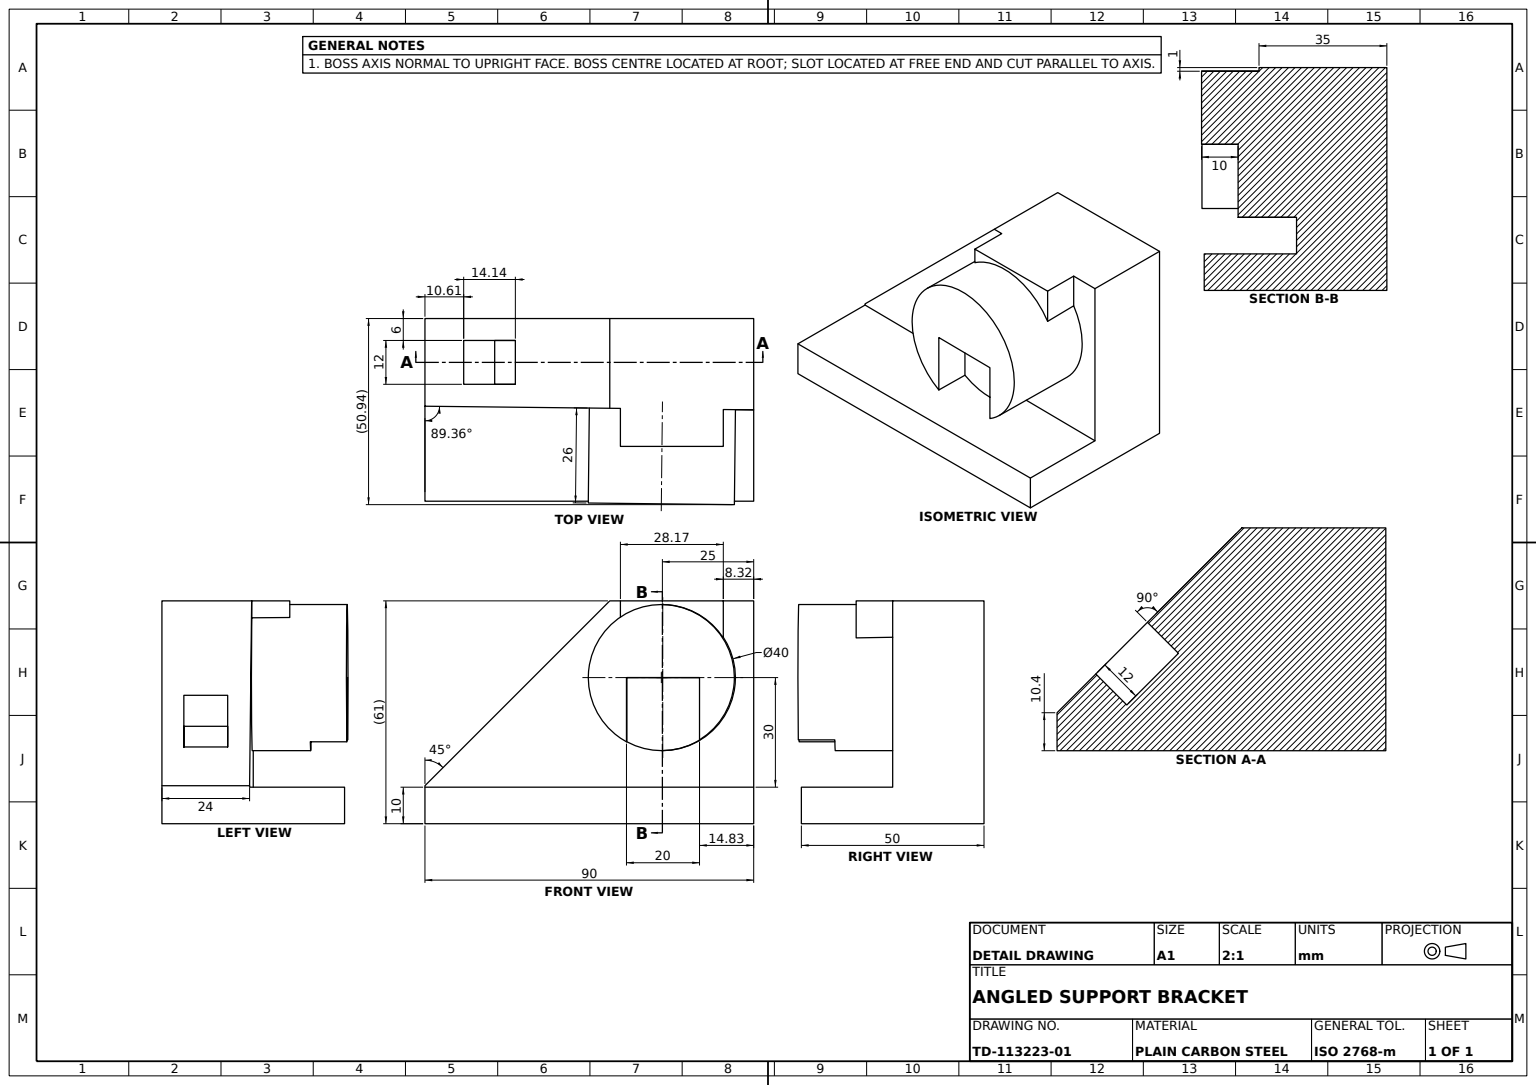
SolidWorks part; units mm, degrees
material "Plain Carbon Steel"
ref_plane "Front Plane" through (0, 0, 0) normal (0, 0, 1) x (1, 0, 0)
ref_plane "Top Plane" through (0, 0, 0) normal (0, 1, 0) x (1, 0, 0)
ref_plane "Right Plane" through (0, 0, 0) normal (1, 0, 0) x (0, 0, -1)
sketch "Base Plate Sketch" plane through (0, 0, 0) normal (0, 1, 0) x (1, 0, 0)
  line L1 (34.558, -45) -> (-15.442, -45)
  line L2 (34.558, -45) -> (34.558, 45)
  line L3 (34.558, 45) -> (-15.442, 45)
  line L4 (-15.442, -45) -> (-15.442, 45)
  point P0 (0, 0)
  dimension "D1" = 90
  dimension "D2" = 50
  dimension "D3" = 15.442
  dimension "D4" = 45
extrude "Base Plate 90x50x10" add sketch "Base Plate Sketch" along normal blind 10
sketch "Upright Block Sketch" plane through (0, 10, 0) normal (0, 1, 0) x (1, 0, 0)
  line L0 (-15.442, -45) -> (8.558, -45)
  line L1 (-15.442, 45) -> (-15.442, -45) construction
  line L2 (-15.442, -45) -> (34.558, -45) construction
  line L3 (8.558, -45) -> (9.558, 45)
  line L4 (34.558, 45) -> (-15.442, 45) construction
  line L5 (9.558, 45) -> (-15.442, 45)
  line L6 (-15.442, 45) -> (-15.442, -45)
  dimension "D1" = 24
extrude "Upright Block" add sketch "Upright Block Sketch" along normal blind 50
sketch "Cylindrical Boss Sketch" plane through (9.0569, 0, 0.1006) normal (0.9999, 0, 0.0111) x (0.0111, 0, -0.9999)
  line L0 (45.1034, 60) -> (45.1034, 10) construction
  line L1 (-44.9021, 10) -> (45.1034, 10) construction
  circle A1 centre (20.1034, 40) radius 20
  dimension "D3" = 30
  dimension "D1" = 40
  dimension "D2" = 25
extrude "Cylindrical Boss" add sketch "Cylindrical Boss Sketch" along normal blind 26
sketch "Boss Slot Sketch" plane through (35.0553, 0, 0.3895) normal (0.9999, 0, 0.0111) x (0.0111, 0, -0.9999)
  line L0 (10.5587, 40) -> (30.5587, 40)
  line L2 (10.5587, 40) -> (10.5587, 19.8034)
  line L3 (30.5587, 40) -> (30.5587, 19.8034)
  circle A0 centre (20.1034, 40) radius 20 construction
  arc A2 (10.5587, 19.8034) -> (30.5587, 19.8034) centre (20.5587, 40) ccw
  point P4 (20.5587, 40)
  dimension "D4" = 20.1966
  dimension "D2" = 22.5367
  dimension "D1" = 20
  dimension "D3" = 0.4553
extrude "Boss Slot 20mm" cut sketch "Boss Slot Sketch" against normal blind 10
sketch "Stepped Boss Sketch" plane through (0, 60, 0) normal (0, 1, 0) x (1, 0, 0)
  line L0 (8.7195, 45) -> (-15.442, 45)
  line L1 (9.558, 45) -> (-15.442, 45) construction
  line L2 (-15.442, 45) -> (-15.442, -45) construction
  line L3 (-15.442, 45) -> (-15.442, -5)
  line L4 (-15.442, -5) -> (9.0025, -5)
  line L5 (8.558, -45) -> (9.2803, 20.0015) construction
  line L6 (9.0025, -5) -> (9.1525, 8.5081)
  line L7 (9.058, 0.0028) -> (9.5025, 40.0003) construction
  line L8 (9.1525, 8.5081) -> (19.558, 8.5081)
  line L9 (19.558, 8.5081) -> (19.558, 36.6775)
  line L10 (19.558, 36.6775) -> (9.4655, 36.6775)
  line L11 (9.2803, 20.0015) -> (9.558, 45) construction
  line L12 (9.4655, 36.6775) -> (9.558, 45)
  line L18 (-15.442, 45) -> (-15.442, -45)
  line L19 (-15.442, -45) -> (8.558, -45)
  line L20 (8.558, -45) -> (9.2803, 20.0015)
  line L21 (9.2803, 20.0015) -> (9.558, 45)
  line L22 (9.558, 45) -> (-15.442, 45)
  line L27 (9.558, 45) -> (8.7195, 45)
  dimension "D1" = 50
  dimension "D2" = 35
  dimension "D4" = 24.1615
  dimension "D5" = 24.5945
  dimension "D6" = 24.9075
  dimension "D3" = 0
extrude "Stepped Boss" add sketch "Stepped Boss Sketch" along normal blind 1 and the other way blind 20
chamfer "Upright Chamfer 10mm" distance 10 angle 45 1 edges at (-3.442, 60, 45)
ref_plane "Angled Cut Plane" through (0, 27.701, 27.701) normal (0, 0.7071, 0.7071) x (1, 0, 0)
sketch "Angled Face Cut Sketch" plane through (0, 27.701, 27.701) normal (0, 0.7071, 0.7071) x (1, 0, 0)
  line L0 (-15.442, 49.3042) -> (9.1661, 49.3042)
  line L1 (-15.442, 38.8909) -> (-15.442, 17.6777) construction
  line L2 (8.6691, 17.6777) -> (9.0025, 38.8909) construction
  line L3 (9.1661, 49.3042) -> (9.1661, -79.3513)
  line L4 (9.1661, -79.3513) -> (-15.442, -79.3513)
  line L5 (-15.442, -79.3513) -> (-15.442, 49.3042)
  dimension "D1" = 24.6081
  dimension "D2" = 128.6555
extrude "Angled Face Cut" cut sketch "Angled Face Cut Sketch" along normal blind 38
ref_plane "Angled Face Plane" through (0, 27.701, 27.701) normal (0, 0.7071, 0.7071) x (1, 0, 0)
sketch "Window Pocket Sketch" plane through (0, 27.701, 27.701) normal (0, 0.7071, 0.7071) x (1, 0, 0)
  line L0 (9.1202, 47.0919) -> (8.558, -24.4645) construction
  line L1 (-9.442, -9.4645) -> (2.558, -9.4645)
  line L2 (-9.442, -9.4645) -> (-9.442, 10.5355)
  line L3 (-9.442, 10.5355) -> (2.558, 10.5355)
  line L4 (2.558, -9.4645) -> (2.558, 10.5355)
  line L5 (8.558, -24.4645) -> (-15.442, -24.4645) construction
  line L6 (-15.442, 47.0919) -> (-15.442, -24.4645) construction
  dimension "D1" = 0.45
  dimension "D2" = 12
  dimension "D3" = 20
  dimension "D4" = 15
  dimension "D5" = 6
extrude "Rectangular Window Pocket" cut sketch "Window Pocket Sketch" against normal blind 12
